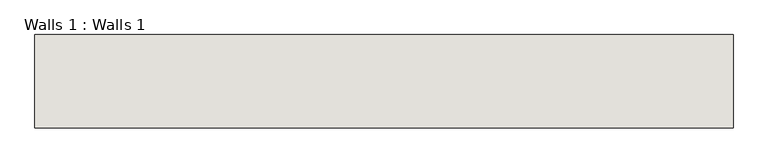
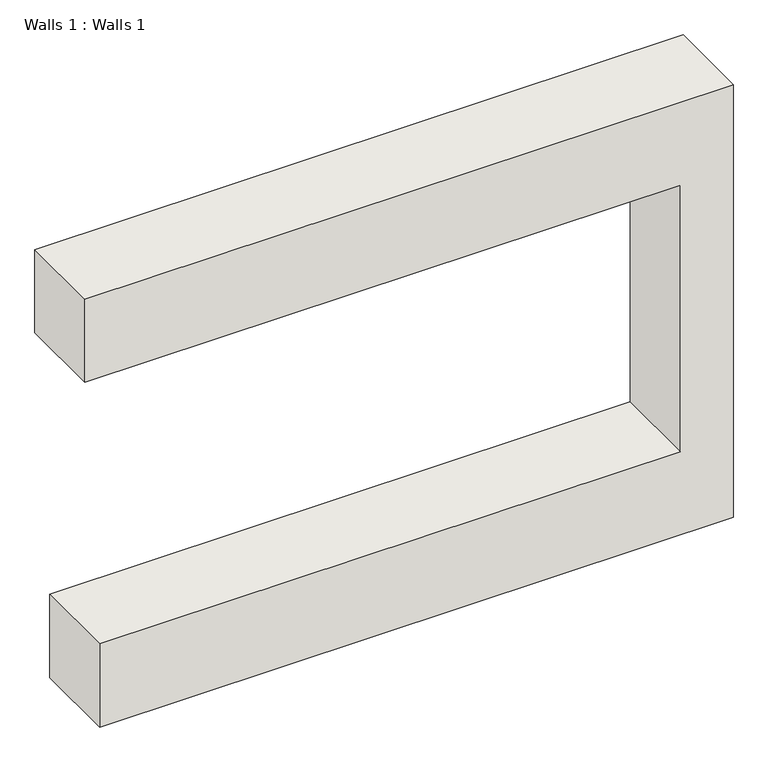
"""IFC4 building model written with IfcOpenShell, lengths in millimetres: wall geometry, Walls 1 : Walls 1."""

from ifc_helpers import new_model, si_unit, frame, origin, place, context, project, spatial, polyline, outline, extrude, source, transform, mapped, element, save


def walls_1_walls_1_5292a9a1(model_context):
    return source(origin(), model_context, "Body", "SweptSolid", [
        extrude(outline(polyline([(11277.6, -4247.9432037), (11277.6, -9861.3432037), (10515.6, -9861.3432037), (10515.6, -4705.1432037), (8077.2, -4705.1432037), (8077.2, -9734.3432037), (7315.2, -9734.3432037), (7315.2, -4247.9432037), (11277.6, -4247.9432037)])), frame((0.0, 497.9548476, 0.0), z_axis=(0.0, 1.0, 0.0), x_axis=(0.0, 0.0, 1.0)), (0.0, 0.0, 1.0), 749.3000267),
    ])


if __name__ == "__main__":
    model = new_model("IFC4")
    model_context = context("Model", 3, world=origin())
    ifc_project = project(units=[si_unit("LENGTHUNIT", "METRE", prefix="MILLI")], contexts=[model_context])
    site = spatial("IfcSite", under=ifc_project)
    building = spatial("IfcBuilding", under=site)
    placement = place(None, origin())
    walls_1_walls_1_shape = walls_1_walls_1_5292a9a1(model_context)
    element("IfcWall", 1, ObjectType="Walls 1 : Walls 1", at=placement, inside=building, context=model_context, shape_type="MappedRepresentation", body=[
        mapped(walls_1_walls_1_shape, transform((0.0, 0.0, 0.0), x_axis=(1.0, 0.0, 0.0), y_axis=(0.0, 1.0, 0.0), z_axis=(0.0, 0.0, 1.0))),
    ])
    save(model, "model.ifc")

# Revit data of these elements
# Element 1 (IfcWall, "Walls 1 : Walls 1")
#   Materials on its faces: "Default Wall"
# Materials
#   "Default Wall": colour RGB 128 128 128, transparency 0
